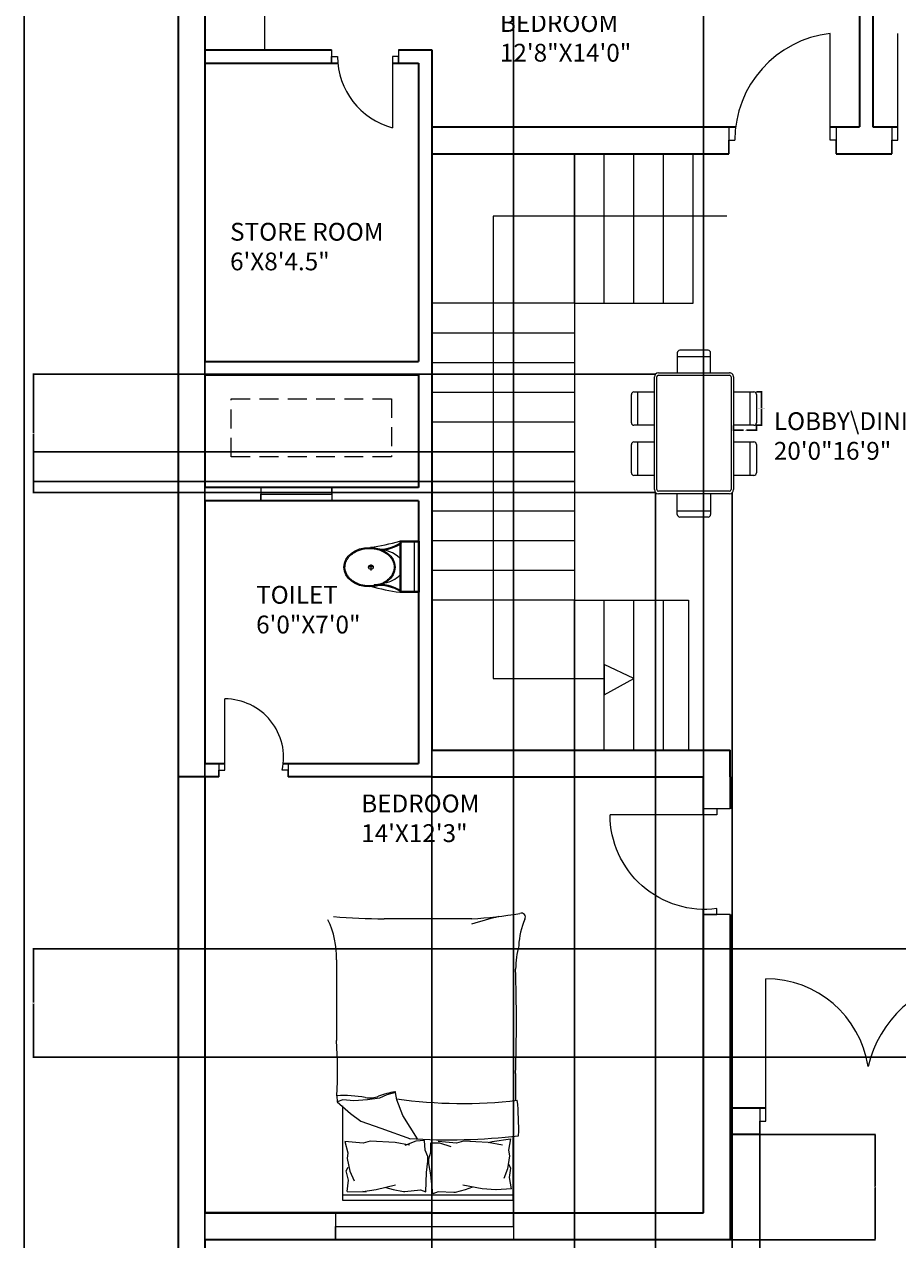
# Model space of a CAD drawing. Units: inches. Extents: x 2460 to 3031, y 933 to 2010.
# Tile 5 of 7: x 2460 to 2754, y 1339 to 1749. Entities that reach past the tile are written whole.
import ezdxf

# ---------------------------------------------------------------- set-up
doc = ezdxf.new("R2010")
doc.units = ezdxf.units.IN
doc.linetypes.add('DASHED2', pattern=[9.525, 6.35, -3.175])
for name, color, linetype, lineweight in [('A-ANNO-DIMS', 2, 'Continuous', 18), ('A-ANNO-SYMB', 7, 'Continuous', 13), ('A-ANNO-TTLB', 7, 'Continuous', 25), ('A-AREA-IDEN', 7, 'Continuous', 18), ('A-DOOR', 4, 'Continuous', 18), ('A-FLOR-CASE', 9, 'Continuous', 18), ('A-FLOR-FIXT', 8, 'Continuous', 18), ('A-FLOR-OVHD', 254, 'DASHED2', 13), ('A-FLOR-STRS', 7, 'Continuous', 18), ('A-FURN', 8, 'Continuous', 18), ('A-GLAZ', 4, 'Continuous', 18), ('A-WALL', 7, 'Continuous', 35), ('C-PROP', 7, 'Continuous', 35)]:
    doc.layers.add(name, color=color, linetype=linetype, lineweight=lineweight)
doc.styles.get("Standard").update_dxf_attribs({"font": 'arial.ttf'})
doc.dimstyles.get("Standard").update_dxf_attribs({"dimtxt": 0.18, "dimasz": 0.18, "dimexe": 0.18, "dimexo": 0.0625, "dimgap": 0.09, "dimtad": 0, "dimtih": 1, "dimtoh": 1, "dimdec": 4, "dimzin": 0, "dimdsep": 46, "dimtxsty": 'Standard', "dimcen": 0.09, "dimadec": 0, "dimazin": 0, "dimtfac": 1, "dimtdec": 4, "dimtofl": 0, "dimtmove": 0, "dimatfit": 3, "dimfxl": 1, "dimtolj": 1, "dimtzin": 0, "dimarcsym": 0})

# ---------------------------------------------------------------- blocks, each defined once
blk = doc.blocks.new('A$C31115884')
for p, q in [((283, 498), (223, 498)), ((258, 466), (258, 523)), ((0, 200), (0, 0)), ((520, 200), (0, 200)), ((10, 190), (10, 10)), ((510, 190), (10, 190)), ((510, 10), (510, 190)), ((520, 0), (520, 200)), ((510, 54), (0, 54)), ((10, 10), (510, 10)), ((0, 0), (520, 0))]:
    blk.add_line(p, q)
blk.add_circle((256, 496), 23.6)
for centre, radius, start, end in [((2778, -205), 2807, 165.4549, 171.7133), ((3237, 905), 2807, 188.2867, 194.5451), ((-295, 403), 365, 324.2091, 9.3499), ((-295, 403), 375, 324.2091, 9.3499), ((139, 406), 293, 315.8436, 2.6563), ((806, 403), 375, 179.2036, 215.7909), ((806, 403), 365, 170.6501, 215.7909), ((384, 406), 293, 190.2774, 224.1564)]:
    blk.add_arc(centre, radius, start, end)
blk.add_ellipse((256, 510), major_axis=(0, -261), ratio=0.772727)
blk.add_open_spline([(256, 259), (263, 259), (270, 260), (288, 262), (299, 265), (320, 273), (330, 278), (350, 291), (360, 299), (378, 316), (386, 326), (402, 347), (409, 358), (421, 383), (427, 395), (436, 422), (440, 436), (445, 465), (447, 480), (448, 509), (448, 524), (445, 553), (443, 568), (436, 596), (432, 610), (422, 636), (416, 649), (402, 672), (395, 683), (379, 703), (370, 712), (351, 728), (341, 735), (321, 746), (310, 751), (289, 757), (278, 759), (256, 761), (245, 761), (223, 757), (212, 754), (191, 746), (181, 741), (161, 728), (151, 720), (133, 703), (125, 693), (110, 672), (103, 660), (90, 636), (85, 623), (76, 596), (72, 582), (67, 553), (66, 538), (64, 509), (65, 494), (68, 465), (70, 450), (77, 422), (81, 408), (91, 382), (97, 370), (111, 346), (118, 335), (135, 316), (144, 307), (162, 291), (172, 284), (193, 273), (203, 269), (225, 262), (236, 260), (250, 259), (253, 259), (256, 259)], degree=3, knots=[0, 0, 0, 0, 0.110105, 0.110105, 0.285049, 0.285049, 0.459994, 0.459994, 0.634938, 0.634938, 0.809882, 0.809882, 0.984827, 0.984827, 1.159771, 1.159771, 1.334715, 1.334715, 1.50966, 1.50966, 1.684604, 1.684604, 1.859549, 1.859549, 2.034493, 2.034493, 2.209437, 2.209437, 2.384382, 2.384382, 2.559326, 2.559326, 2.73427, 2.73427, 2.909215, 2.909215, 3.084159, 3.084159, 3.259103, 3.259103, 3.434048, 3.434048, 3.608992, 3.608992, 3.783936, 3.783936, 3.958881, 3.958881, 4.133825, 4.133825, 4.30877, 4.30877, 4.483714, 4.483714, 4.658658, 4.658658, 4.833603, 4.833603, 5.008547, 5.008547, 5.183491, 5.183491, 5.358436, 5.358436, 5.53338, 5.53338, 5.708324, 5.708324, 5.883269, 5.883269, 6.058213, 6.058213, 6.233158, 6.233158, 6.283185, 6.283185, 6.283185, 6.283185])
blk = doc.blocks.new('BED-DOUBLE')
for p, q in [((75.16, 62.38), (96.87, 62.38)), ((76.95, 55.42), (76.08, 61.53)), ((76.08, 61.53), (79.9, 60.84)), ((85.96, 61.71), (84.75, 61.01)), ((89.08, 61.19), (85.96, 61.71)), ((92.9, 61.88), (89.08, 61.19)), ((92.87, 61.87), (93.27, 56.74)), ((95.03, 62.38), (95.03, 5.09)), ((96.87, 62.38), (96.87, 5.09)), ((78.14, 58.9), (77.34, 54.06)), ((79.9, 60.84), (81.8, 61.19)), ((81.8, 61.19), (86.14, 60.49)), ((86.14, 60.49), (89.43, 59.28)), ((77.34, 54.06), (76.82, 45.66)), ((77.34, 54.06), (76.95, 55.42)), ((93.24, 56.62), (92.9, 52.03)), ((93.27, 56.74), (93.24, 56.62)), ((92.9, 52.03), (91.68, 45.45)), ((1.87, 48.49), (1.87, 18.98)), ((76.82, 45.66), (77.49, 43.31)), ((92.38, 48.74), (93.24, 46.31)), ((93.24, 46.31), (94.11, 42.85)), ((77.49, 43.31), (77, 37.16)), ((77.37, 37.65), (78.68, 41.42)), ((94.11, 42.46), (93.94, 37.13)), ((94.11, 42.85), (94.11, 42.46)), ((77.37, 34.71), (77.37, 37.65)), ((93.94, 37.13), (94.63, 35.4)), ((79.83, 32.82), (76.62, 32.62)), ((80.59, 34.71), (77.37, 34.71)), ((82.03, 33.66), (79.83, 32.82)), ((82.84, 34.01), (80.59, 34.71)), ((83.59, 33.75), (82.03, 33.66)), ((84.4, 34.01), (82.84, 34.01)), ((87.44, 33.3), (83.59, 33.75)), ((88.22, 34.71), (84.4, 34.01)), ((93.88, 33.01), (87.44, 33.3)), ((94.63, 35.4), (88.22, 34.71)), ((93.3, 31.24), (93.88, 33.01)), ((76.03, 30.27), (68.25, 25.25)), ((76.62, 32.62), (76.8, 29.68)), ((76.8, 29.68), (78.34, 26)), ((93.81, 25.93), (93.3, 31.24)), ((68.25, 25.25), (62.87, 23.21)), ((72.52, 17.82), (76.03, 27.82)), ((78.14, 27.51), (77.34, 22.68)), ((93.18, 22.03), (93.83, 25.54)), ((93.83, 25.54), (93.81, 25.93)), ((62.87, 23.21), (60.45, 22.84)), ((60.45, 22.84), (61.2, 19.86)), ((77.34, 22.68), (76.82, 14.27)), ((93.19, 16.3), (91.57, 22.8)), ((92.47, 19.55), (93.18, 22.03)), ((61.2, 19.86), (62.31, 17.45)), ((62.31, 17.45), (62.87, 13.37)), ((70.1, 11.14), (72.52, 17.82)), ((62.87, 13.37), (63.24, 8.72)), ((76.82, 14.27), (77.49, 11.92)), ((93.82, 11.75), (93.19, 16.3)), ((93.81, 6.47), (93.92, 12.95)), ((93.92, 12.95), (93.82, 11.75)), ((63.24, 8.72), (62.87, 5.01)), ((67.51, 7.61), (70.1, 11.14)), ((77.49, 11.92), (77, 5.77)), ((86.97, 7.43), (90.18, 8.85)), ((62.87, 5.01), (63.61, 3.17)), ((63.61, 3.17), (67.51, 7.61)), ((96.87, 5.09), (64.97, 5.09)), ((77, 5.77), (80.77, 6.7)), ((80.77, 6.7), (82.69, 6.47)), ((82.69, 6.47), (86.97, 7.43)), ((86.88, 6.21), (85.62, 6.83)), ((89.96, 6.93), (86.88, 6.21)), ((93.81, 6.47), (89.96, 6.93)), ((61.52, 3.07), (63.61, 3.17, 4.64))]:
    blk.add_line(p, q)
for centre, radius, start, end in [((1.3, 65.24), 1.31, 56.1736, 203.4781), ((12.62, 92.52), 28.25, 247.9751, 266.652), ((-143.9, 40.86), 145.97, 2.9958, 9.4091), ((19.53, 98.8), 35.53, 256.0648, 268.9113), ((36.19, -514.68), 578.22, 88.22771, 91.71854), ((59.5, 267.13), 203.94, 268.4762, 271.0082), ((-90.53, 45.26), 154.68, 351.7845, 6.9006), ((72.78, -35.55), 99.87, 88.7218, 95.604), ((-121.38, 40.94), 197.77, 356.0865, 6.7821), ((125.3, 87.2), 127.63, 193.3832, 197.7053), ((60.38, 22.63), 0.221, 70.2464, 181.1377), ((95.1, 29.2), 35.55, 190.6617, 199.8806), ((-157.62, 17.21), 159.5, 354.4998, 0.6351), ((54.83, 14.11), 7.46, 348.6608, 23.7384), ((104.85, 5.01), 43.38, 169.8763, 182.5657), ((14.55, -24.75), 27.65, 87.4714, 116.4681), ((15.56, 5471.89), 5469.02, 270.00217, 270.28689), ((53.34, -151.96), 155.25, 86.9791, 93.8365)]:
    blk.add_arc(centre, radius, start, end)
blk = doc.blocks.new('CHAIR-DINING-SIDE')
for p, q in [((0, 11.24), (6.88, 11.24)), ((5.62, 0), (5.62, 11.24)), ((7.73, 10.4), (7.73, 0.84)), ((6.88, 0), (0, 0))]:
    blk.add_line(p, q)
for centre, start, end in [((6.88, 10.4), 0, 90), ((6.88, 0.84), 270, 0)]:
    blk.add_arc(centre, 0.843, start, end)
blk = doc.blocks.new('DOOR-SWING-36')
for p, q in [((0, 35.65), (9, 35.65)), ((4.5, 35.65), (4.5, 33.65)), ((4.5, 33.65), (40.5, 33.65)), ((4.5, 0), (4.5, 2)), ((0, 0), (9, 0)), ((9, 0), (4.5, 0))]:
    blk.add_line(p, q)
blk.add_arc((8.58, 33.65), 31.92, 262.6481, 0)
blk = doc.blocks.new('WIN-24-PARTITION')
for p, q in [((2.25, 24), (0, 24)), ((0, 24), (4.5, 24)), ((2.25, 0), (2.25, 24)), ((0, 0), (4.5, 0)), ((4.5, 0), (2.25, 0))]:
    blk.add_line(p, q)
blk = doc.blocks.new('WIN-60')
for p, q in [((0, 9), (0, 0)), ((60, 4.5), (60, 9)), ((60, 9), (60, 0)), ((0, 0), (0, 4.5)), ((0, 4.5), (60, 4.5))]:
    blk.add_line(p, q)
blk = doc.blocks.new('*D16')
at = {"layer": 'A-ANNO-DIMS', "color": 0, "lineweight": -2, "transparency": 16777216}
for p, q in [((2706.57, 1625.17), (2708.38, 1625.17)), ((2708.2, 1624.99), (2708.2, 1619.74)), ((2708.2, 1614.12), (2708.2, 1619.37)), ((2706.57, 1613.94), (2708.38, 1613.94))]:
    blk.add_line(p, q, dxfattribs=at)
at = {"layer": 'A-ANNO-DIMS', "color": 0, "transparency": 16777216}
for points in [[(2708.17, 1624.99), (2708.23, 1624.99), (2708.2, 1625.17)], [(2708.17, 1614.12), (2708.23, 1614.12), (2708.2, 1613.94)]]:
    blk.add_solid(points, dxfattribs=at)
at = {"layer": 'Defpoints', "color": 0, "transparency": 16777216}
for p in [(2706.51, 1625.17), (2708.2, 1625.17), (2706.51, 1613.94)]:
    blk.add_point(p, dxfattribs=at)
at = {"layer": 'A-ANNO-DIMS', "color": 0, "transparency": 16777216, "insert": (2708.2, 1619.55), "char_height": 0.18, "attachment_point": 5}
blk.add_mtext('\\A1;SIDE CHAIR 11 TYP.', dxfattribs=at)
blk = doc.blocks.new('*D17')
at = {"layer": 'A-ANNO-DIMS', "color": 0, "lineweight": -2, "transparency": 16777216}
for p, q in [((2698.78, 1613.87), (2698.78, 1612.07)), ((2706.51, 1613.87), (2706.51, 1612.07)), ((2698.96, 1612.25), (2702.19, 1612.25)), ((2706.33, 1612.25), (2703.11, 1612.25))]:
    blk.add_line(p, q, dxfattribs=at)
at = {"layer": 'A-ANNO-DIMS', "color": 0, "transparency": 16777216}
for points in [[(2698.96, 1612.28), (2698.96, 1612.22), (2698.78, 1612.25)], [(2706.33, 1612.28), (2706.33, 1612.22), (2706.51, 1612.25)]]:
    blk.add_solid(points, dxfattribs=at)
at = {"layer": 'Defpoints', "color": 0, "transparency": 16777216}
for p in [(2698.78, 1613.94), (2706.51, 1613.94), (2706.51, 1612.25)]:
    blk.add_point(p, dxfattribs=at)
at = {"layer": 'A-ANNO-DIMS', "color": 0, "transparency": 16777216, "insert": (2702.65, 1612.25), "char_height": 0.18, "attachment_point": 5}
blk.add_mtext('\\A1;8 TYP.', dxfattribs=at)
blk = doc.blocks.new('*D37')
at = {"layer": 'A-ANNO-DIMS', "color": 0, "lineweight": -2, "transparency": 16777216}
for p, q in [((2597.17, 1554.98), (2597.17, 933.16)), ((2645.17, 1554.98), (2645.17, 933.16)), ((2597.35, 933.34), (2620.95, 933.34)), ((2644.99, 933.34), (2621.39, 933.34))]:
    blk.add_line(p, q, dxfattribs=at)
at = {"layer": 'A-ANNO-DIMS', "color": 0, "transparency": 16777216}
for points in [[(2597.35, 933.37), (2597.35, 933.31), (2597.17, 933.34)], [(2644.99, 933.37), (2644.99, 933.31), (2645.17, 933.34)]]:
    blk.add_solid(points, dxfattribs=at)
at = {"layer": 'Defpoints', "color": 0, "transparency": 16777216}
for p in [(2597.17, 1555.05), (2645.17, 1555.05), (2645.17, 933.34)]:
    blk.add_point(p, dxfattribs=at)
at = {"layer": 'A-ANNO-DIMS', "color": 0, "transparency": 16777216, "insert": (2621.17, 933.34), "char_height": 0.18, "attachment_point": 5}
blk.add_mtext('\\A1;48', dxfattribs=at)
blk = doc.blocks.new('*D38')
at = {"layer": 'A-ANNO-DIMS', "color": 0, "lineweight": -2, "transparency": 16777216}
for p, q in [((2672.51, 1591.25), (2672.51, 933.16)), ((2698.37, 1591.25), (2698.37, 933.16)), ((2672.69, 933.34), (2685.04, 933.34)), ((2698.19, 933.34), (2685.83, 933.34))]:
    blk.add_line(p, q, dxfattribs=at)
at = {"layer": 'A-ANNO-DIMS', "color": 0, "transparency": 16777216}
for points in [[(2672.69, 933.37), (2672.69, 933.31), (2672.51, 933.34)], [(2698.19, 933.37), (2698.19, 933.31), (2698.37, 933.34)]]:
    blk.add_solid(points, dxfattribs=at)
at = {"layer": 'Defpoints', "color": 0, "transparency": 16777216}
for p in [(2672.51, 1591.31), (2698.37, 1591.31), (2698.37, 933.34)]:
    blk.add_point(p, dxfattribs=at)
at = {"layer": 'A-ANNO-DIMS', "color": 0, "transparency": 16777216, "insert": (2685.44, 933.34), "char_height": 0.18, "attachment_point": 5}
blk.add_mtext('\\A1;25.87', dxfattribs=at)
blk = doc.blocks.new('*D39')
at = {"layer": 'A-ANNO-DIMS', "color": 0, "lineweight": -2, "transparency": 16777216}
for p, q in [((2672.44, 1631.22), (2462.69, 1631.22)), ((2462.87, 1631.04), (2462.87, 1611.45)), ((2462.87, 1591.49), (2462.87, 1611.08)), ((2672.44, 1591.31), (2462.69, 1591.31))]:
    blk.add_line(p, q, dxfattribs=at)
at = {"layer": 'A-ANNO-DIMS', "color": 0, "transparency": 16777216}
for points in [[(2462.84, 1631.04), (2462.9, 1631.04), (2462.87, 1631.22)], [(2462.84, 1591.49), (2462.9, 1591.49), (2462.87, 1591.31)]]:
    blk.add_solid(points, dxfattribs=at)
at = {"layer": 'Defpoints', "color": 0, "transparency": 16777216}
for p in [(2462.87, 1631.22), (2672.51, 1631.22), (2672.51, 1591.31)]:
    blk.add_point(p, dxfattribs=at)
at = {"layer": 'A-ANNO-DIMS', "color": 0, "transparency": 16777216, "insert": (2462.87, 1611.27), "char_height": 0.18, "attachment_point": 5}
blk.add_mtext('\\A1;39.92', dxfattribs=at)
blk = doc.blocks.new('*D40')
at = {"layer": 'A-ANNO-DIMS', "color": 0, "lineweight": -2, "transparency": 16777216}
for p, q in [((2511.67, 1056.05), (2511.67, 2006.96)), ((2511.85, 2006.78), (2516.02, 2006.78)), ((2520.49, 2006.78), (2516.32, 2006.78)), ((2520.67, 1056.05), (2520.67, 2006.96))]:
    blk.add_line(p, q, dxfattribs=at)
at = {"layer": 'A-ANNO-DIMS', "color": 0, "transparency": 16777216}
for points in [[(2511.85, 2006.81), (2511.85, 2006.75), (2511.67, 2006.78)], [(2520.49, 2006.81), (2520.49, 2006.75), (2520.67, 2006.78)]]:
    blk.add_solid(points, dxfattribs=at)
at = {"layer": 'Defpoints', "color": 0, "transparency": 16777216}
for p in [(2520.67, 2006.78), (2511.67, 1055.98), (2520.67, 1055.98)]:
    blk.add_point(p, dxfattribs=at)
at = {"layer": 'A-ANNO-DIMS', "color": 0, "transparency": 16777216, "insert": (2516.17, 2006.78), "char_height": 0.18, "attachment_point": 5}
blk.add_mtext('\\A1;9', dxfattribs=at)
blk = doc.blocks.new('*D42')
at = {"layer": 'A-ANNO-DIMS', "color": 0, "lineweight": -2, "transparency": 16777216}
for p, q in [((2645.11, 1605.05), (2462.69, 1605.05)), ((2462.87, 1604.87), (2462.87, 1600.23)), ((2462.87, 1595.23), (2462.87, 1599.86)), ((2645.11, 1595.05), (2462.69, 1595.05))]:
    blk.add_line(p, q, dxfattribs=at)
at = {"layer": 'A-ANNO-DIMS', "color": 0, "transparency": 16777216}
for points in [[(2462.84, 1604.87), (2462.9, 1604.87), (2462.87, 1605.05)], [(2462.84, 1595.23), (2462.9, 1595.23), (2462.87, 1595.05)]]:
    blk.add_solid(points, dxfattribs=at)
at = {"layer": 'Defpoints', "color": 0, "transparency": 16777216}
for p in [(2462.87, 1605.05), (2645.17, 1605.05), (2645.17, 1595.05)]:
    blk.add_point(p, dxfattribs=at)
at = {"layer": 'A-ANNO-DIMS', "color": 0, "transparency": 16777216, "insert": (2462.87, 1600.05), "char_height": 0.18, "attachment_point": 5}
blk.add_mtext('\\A1;10', dxfattribs=at)
blk = doc.blocks.new('*D43')
at = {"layer": 'A-ANNO-DIMS', "color": 0, "lineweight": -2, "transparency": 16777216}
for p, q in [((2707.62, 1374.89), (2707.62, 933.16)), ((2778.55, 1374.89), (2778.55, 933.16)), ((2707.8, 933.34), (2742.69, 933.34)), ((2778.37, 933.34), (2743.48, 933.34))]:
    blk.add_line(p, q, dxfattribs=at)
at = {"layer": 'A-ANNO-DIMS', "color": 0, "transparency": 16777216}
for points in [[(2707.8, 933.37), (2707.8, 933.31), (2707.62, 933.34)], [(2778.37, 933.37), (2778.37, 933.31), (2778.55, 933.34)]]:
    blk.add_solid(points, dxfattribs=at)
at = {"layer": 'Defpoints', "color": 0, "transparency": 16777216}
for p in [(2707.62, 1374.95), (2778.55, 1374.95), (2778.55, 933.34)]:
    blk.add_point(p, dxfattribs=at)
at = {"layer": 'A-ANNO-DIMS', "color": 0, "transparency": 16777216, "insert": (2743.09, 933.34), "char_height": 0.18, "attachment_point": 5}
blk.add_mtext('\\A1;70.93', dxfattribs=at)
blk = doc.blocks.new('*D44')
at = {"layer": 'A-ANNO-DIMS', "color": 0, "lineweight": -2, "transparency": 16777216}
for p, q in [((2624.64, 1348.55), (2624.64, 2006.96)), ((2624.82, 2006.78), (2656.26, 2006.78)), ((2688.49, 2006.78), (2657.05, 2006.78)), ((2688.67, 1348.55), (2688.67, 2006.96))]:
    blk.add_line(p, q, dxfattribs=at)
at = {"layer": 'A-ANNO-DIMS', "color": 0, "transparency": 16777216}
for points in [[(2624.82, 2006.81), (2624.82, 2006.75), (2624.64, 2006.78)], [(2688.49, 2006.81), (2688.49, 2006.75), (2688.67, 2006.78)]]:
    blk.add_solid(points, dxfattribs=at)
at = {"layer": 'Defpoints', "color": 0, "transparency": 16777216}
for p in [(2688.67, 2006.78), (2624.64, 1348.48), (2688.67, 1348.48)]:
    blk.add_point(p, dxfattribs=at)
at = {"layer": 'A-ANNO-DIMS', "color": 0, "transparency": 16777216, "insert": (2656.65, 2006.78), "char_height": 0.18, "attachment_point": 5}
blk.add_mtext('\\A1;64.03', dxfattribs=at)
blk = doc.blocks.new('*D50')
at = {"layer": 'A-ANNO-DIMS', "color": 0, "lineweight": -2, "transparency": 16777216}
for p, q in [((2901.55, 1437.46), (2462.69, 1437.46)), ((2462.87, 1437.28), (2462.87, 1419.38)), ((2462.87, 1401.12), (2462.87, 1419.02)), ((2901.55, 1400.94), (2462.69, 1400.94))]:
    blk.add_line(p, q, dxfattribs=at)
at = {"layer": 'A-ANNO-DIMS', "color": 0, "transparency": 16777216}
for points in [[(2462.84, 1437.28), (2462.9, 1437.28), (2462.87, 1437.46)], [(2462.84, 1401.12), (2462.9, 1401.12), (2462.87, 1400.94)]]:
    blk.add_solid(points, dxfattribs=at)
at = {"layer": 'Defpoints', "color": 0, "transparency": 16777216}
for p in [(2462.87, 1437.46), (2901.62, 1437.46), (2901.62, 1400.94)]:
    blk.add_point(p, dxfattribs=at)
at = {"layer": 'A-ANNO-DIMS', "color": 0, "transparency": 16777216, "insert": (2462.87, 1419.2), "char_height": 0.18, "attachment_point": 5}
blk.add_mtext('\\A1;36.524', dxfattribs=at)
blk = doc.blocks.new('*D51')
at = {"layer": 'A-ANNO-DIMS', "color": 0, "lineweight": -2, "transparency": 16777216}
for p, q in [((2697.73, 1374.95), (2746.65, 1374.95)), ((2746.47, 1374.77), (2746.47, 1357.4)), ((2746.47, 1339.66), (2746.47, 1357.03)), ((2697.73, 1339.48), (2746.65, 1339.48))]:
    blk.add_line(p, q, dxfattribs=at)
at = {"layer": 'A-ANNO-DIMS', "color": 0, "transparency": 16777216}
for points in [[(2746.44, 1374.77), (2746.5, 1374.77), (2746.47, 1374.95)], [(2746.44, 1339.66), (2746.5, 1339.66), (2746.47, 1339.48)]]:
    blk.add_solid(points, dxfattribs=at)
at = {"layer": 'Defpoints', "color": 0, "transparency": 16777216}
for p in [(2697.67, 1374.95), (2697.67, 1339.48), (2746.47, 1339.48)]:
    blk.add_point(p, dxfattribs=at)
at = {"layer": 'A-ANNO-DIMS', "color": 0, "transparency": 16777216, "insert": (2746.47, 1357.22), "char_height": 0.18, "attachment_point": 5}
blk.add_mtext('\\A1;35.466', dxfattribs=at)

msp = doc.modelspace()

# ---------------------------------------------------------------- linework, layer by layer
at = {"layer": 'A-ANNO-SYMB'}
for p, q in [((2696.5623, 1684.4614), (2617.8347, 1684.4614)), ((2617.8347, 1684.4614), (2617.8347, 1528.6315)), ((2665.1684, 1528.6315), (2655.1684, 1533.301)), ((2655.1684, 1533.301), (2655.1684, 1523.12)), ((2617.8347, 1528.6315), (2655.1684, 1528.6315)), ((2655.1684, 1523.12), (2665.1684, 1528.6315))]:
    msp.add_line(p, q, dxfattribs=at)
at = {"layer": 'A-ANNO-TTLB'}
msp.add_lwpolyline([(2459.8083, 2009.7942), (3030.6598, 2009.7942), (3030.6598, 936.3732), (2459.8083, 936.3732)], close=True, dxfattribs=at)
at = {"layer": 'A-DOOR'}
for p, q in [((2731.3312, 1709.9828), (2731.3312, 1745.9828)), ((2754.0876, 1709.9828), (2754.0876, 1745.9828)), ((2563.3673, 1740.4828), (2563.3673, 1735.9828)), ((2563.3673, 1735.9828), (2563.3673, 1738.2328)), ((2563.3673, 1738.2328), (2565.3673, 1738.2328)), ((2585.907, 1738.2328), (2583.907, 1738.2328)), ((2583.907, 1738.2328), (2583.907, 1714.2328)), ((2585.907, 1740.4828), (2585.907, 1735.9828)), ((2585.907, 1735.9828), (2585.907, 1738.2328)), ((2697.2049, 1714.4828), (2697.2049, 1705.4828)), ((2733.3312, 1714.4828), (2733.3312, 1705.4828)), ((2752.0876, 1714.4828), (2752.0876, 1705.4828)), ((2697.2049, 1705.4828), (2697.2049, 1709.9828)), ((2697.2049, 1709.9828), (2699.2049, 1709.9828)), ((2733.3312, 1709.9828), (2731.3312, 1709.9828)), ((2733.3312, 1705.4828), (2733.3312, 1709.9828)), ((2752.0876, 1705.4828), (2752.0876, 1709.9828)), ((2752.0876, 1709.9828), (2754.0876, 1709.9828)), ((2527.3672, 1497.7328), (2527.3672, 1521.7328)), ((2525.3672, 1499.9828), (2525.3672, 1495.4828)), ((2548.7319, 1499.9828), (2548.7319, 1495.4828)), ((2525.3672, 1495.4828), (2525.3672, 1497.7328)), ((2525.3672, 1497.7328), (2527.3672, 1497.7328)), ((2548.7319, 1497.7328), (2546.7319, 1497.7328)), ((2548.7319, 1495.4828), (2548.7319, 1497.7328)), ((2709.6216, 1415.4491), (2709.6216, 1427.4491)), ((2709.6216, 1379.4491), (2709.6216, 1415.4491)), ((2707.6216, 1383.9491), (2707.6216, 1374.9491)), ((2707.6216, 1374.9491), (2707.6216, 1379.4491)), ((2707.6216, 1379.4491), (2709.6216, 1379.4491))]:
    msp.add_line(p, q, dxfattribs=at)
for centre, radius, start, end in [((2735.4384, 1709.9828), 36.2335, 96.508647, 180), ((2590.1713, 1738.2328), 24.8041, 180, 255.371471), ((2527.3672, 1501.9205), 19.8123, 347.797364, 90), ((2709.6216, 1392.5701), 34.879, 8.735664, 90), ((2781.8372, 1389.0544), 38.7565, 97.834609, 166.856265)]:
    msp.add_arc(centre, radius, start, end, dxfattribs=at)
at = {"layer": 'A-FLOR-CASE'}
msp.add_line((2540.7485, 1842.4828), (2540.7485, 1740.4828), dxfattribs=at)
at = {"layer": 'A-FLOR-OVHD'}
msp.add_lwpolyline([(2529.5594, 1622.8177), (2583.5305, 1622.8177), (2583.5305, 1603.3491), (2529.5594, 1603.3491)], close=True, dxfattribs=at)
at = {"layer": 'A-FLOR-STRS'}
for p, q in [((2645.1684, 1705.4828), (2645.1684, 1655.0454)), ((2645.1684, 1655.0454), (2645.1684, 1705.4828)), ((2655.1684, 1655.0454), (2655.1684, 1705.4828)), ((2665.1684, 1655.0454), (2665.1684, 1705.4828)), ((2675.1684, 1655.0454), (2675.1684, 1705.4828)), ((2685.1684, 1655.0454), (2685.1684, 1705.4828)), ((2645.1684, 1655.0454), (2597.1684, 1655.0454)), ((2645.1684, 1657.4828), (2645.1684, 1552.4828)), ((2645.1684, 1655.0454), (2685.1684, 1655.0454)), ((2645.1684, 1645.0454), (2597.1684, 1645.0454)), ((2645.1684, 1635.0454), (2597.1684, 1635.0454)), ((2645.1684, 1625.0454), (2597.1684, 1625.0454)), ((2645.1684, 1615.0454), (2597.1684, 1615.0454)), ((2645.1684, 1605.0454), (2597.1684, 1605.0454)), ((2645.1684, 1595.0454), (2597.1684, 1595.0454)), ((2645.1684, 1585.0454), (2597.1684, 1585.0454)), ((2645.1684, 1575.0454), (2597.1684, 1575.0454)), ((2645.1684, 1565.0454), (2597.1684, 1565.0454)), ((2645.1684, 1555.0454), (2597.1684, 1555.0454)), ((2597.1684, 1504.4828), (2597.1684, 1552.4828)), ((2645.1684, 1555.0454), (2645.1684, 1504.4828)), ((2645.1684, 1504.4828), (2645.1684, 1555.0454)), ((2645.1684, 1555.0454), (2683.6492, 1555.0454)), ((2655.1684, 1504.4828), (2655.1684, 1555.0454)), ((2665.1684, 1504.4828), (2665.1684, 1555.0454)), ((2675.1684, 1504.4828), (2675.1684, 1555.0454)), ((2683.6492, 1555.0454), (2683.6492, 1504.4828))]:
    msp.add_line(p, q, dxfattribs=at)
at = {"layer": 'A-FURN'}
for p, q in [((2690.2157, 1639.2221), (2680.663, 1639.2221)), ((2679.8201, 1638.3792), (2679.8201, 1631.6361)), ((2679.8201, 1637.1148), (2691.0585, 1637.1148)), ((2691.0585, 1631.6361), (2691.0585, 1638.3792)), ((2672.0936, 1592.3014), (2672.0936, 1630.2313)), ((2672.9365, 1592.3014), (2672.9365, 1630.2313)), ((2673.4985, 1631.6361), (2697.3802, 1631.6361)), ((2673.4985, 1630.7932), (2697.3802, 1630.7932)), ((2697.9421, 1630.2313), (2697.9421, 1592.3015)), ((2698.785, 1630.2313), (2698.785, 1592.3015)), ((2697.3802, 1591.7396), (2673.4985, 1591.7396)), ((2697.3802, 1590.8967), (2673.4985, 1590.8967)), ((2679.8201, 1583.8726), (2679.8201, 1590.8967)), ((2691.0585, 1590.8967), (2691.0585, 1583.8726)), ((2679.8201, 1585.137), (2691.0585, 1585.137)), ((2690.2157, 1583.0297), (2680.663, 1583.0297))]:
    msp.add_line(p, q, dxfattribs=at)
for centre, radius, start, end in [((2680.663, 1638.3792), 0.8429, 90, 180), ((2690.2157, 1638.3792), 0.8429, 0, 90), ((2673.4985, 1630.2313), 1.4048, 90.000003, 180), ((2673.4985, 1630.2313), 0.5619, 90.000003, 180), ((2697.3802, 1630.2313), 1.4048, 0, 90.00001), ((2697.3802, 1630.2313), 0.5619, 0, 90.00001), ((2673.4985, 1592.3014), 1.4048, 180, 270), ((2673.4985, 1592.3014), 0.5619, 180, 270), ((2697.3802, 1592.3015), 1.4048, 270, 0), ((2697.3802, 1592.3015), 0.5619, 270, 0), ((2680.663, 1583.8726), 0.8429, 180, 270), ((2690.2157, 1583.8726), 0.8429, 270, 0)]:
    msp.add_arc(centre, radius, start, end, dxfattribs=at)
at = {"layer": 'A-WALL'}
for p, q in [((2741.1684, 1890.4828), (2741.1684, 1714.4828)), ((2745.6684, 1890.4828), (2745.6684, 1714.4828)), ((2520.6684, 1842.4828), (2520.6684, 1635.4828)), ((2520.6684, 1740.4828), (2563.3673, 1740.4828)), ((2585.907, 1740.4828), (2592.6684, 1740.4828)), ((2592.6684, 1740.4828), (2597.1684, 1740.4828)), ((2597.1684, 1740.4828), (2597.1684, 1504.4828)), ((2520.6684, 1735.9828), (2565.4695, 1735.9828)), ((2583.907, 1735.9828), (2592.6684, 1735.9828)), ((2592.6684, 1735.9828), (2592.6684, 1635.4828)), ((2597.1684, 1714.4828), (2699.4854, 1714.4828)), ((2731.3312, 1714.4828), (2741.1684, 1714.4828)), ((2745.6684, 1714.4828), (2754.0876, 1714.4828)), ((2597.1684, 1705.4828), (2697.2049, 1705.4828)), ((2733.3312, 1705.4828), (2752.0876, 1705.4828)), ((2520.6684, 1635.4828), (2592.6684, 1635.4828)), ((2520.6684, 1630.9828), (2592.6684, 1630.9828)), ((2520.6684, 1630.9828), (2520.6684, 1592.9828)), ((2592.6684, 1630.9828), (2592.6684, 1592.9828)), ((2592.6684, 1592.9828), (2520.6684, 1592.9828)), ((2592.6684, 1588.4828), (2520.6684, 1588.4828)), ((2520.6684, 1588.4828), (2520.6684, 1499.9828)), ((2592.6684, 1588.4828), (2592.6684, 1499.9828)), ((2597.1684, 1504.4828), (2697.6684, 1504.4828)), ((2697.6684, 1495.4828), (2697.6684, 1504.4828)), ((2520.6684, 1499.9828), (2527.3672, 1499.9828)), ((2547.0845, 1499.9828), (2592.6684, 1499.9828)), ((2525.3672, 1495.4828), (2511.6684, 1495.4828)), ((2520.6684, 1495.4828), (2520.6684, 1348.4828)), ((2597.1684, 1495.4828), (2548.7319, 1495.4828)), ((2597.1684, 1495.4828), (2688.6684, 1495.4828)), ((2688.6684, 1482.7065), (2688.6684, 1495.4828)), ((2697.6684, 1495.4828), (2697.6684, 1484.7065)), ((2688.6684, 1348.4828), (2688.6684, 1450.7932)), ((2697.6684, 1449.0529), (2697.6684, 1348.4828)), ((2697.6684, 1383.9491), (2709.6216, 1383.9491)), ((2707.6216, 1374.9491), (2697.6684, 1374.9491)), ((2597.1684, 1348.4828), (2520.6684, 1348.4828)), ((2520.6684, 1348.4828), (2688.6684, 1348.4828)), ((2697.6684, 1348.4828), (2697.6684, 1339.4828)), ((2597.1684, 1339.4828), (2520.6684, 1339.4828)), ((2697.6684, 1339.4828), (2597.1684, 1339.4828))]:
    msp.add_line(p, q, dxfattribs=at)
at = {"layer": 'C-PROP'}
for p, q in [((2511.6684, 1957.9828), (2511.6684, 1055.9828)), ((2511.6684, 1957.9828), (2511.6684, 1055.9828)), ((2520.6684, 1339.4828), (2520.6684, 1055.9828))]:
    msp.add_line(p, q, dxfattribs=at)

# ---------------------------------------------------------------- block references
at = {"layer": 'A-DOOR', "extrusion": (0, 0, -1), "zscale": -1}
msp.add_blockref('DOOR-SWING-36', (-2697.6689, 1449.053), dxfattribs=at)
at = {"layer": 'A-FLOR-FIXT', "xscale": 0.0330640103915726, "yscale": 0.0330640103915726, "zscale": 0.0330640103915726, "rotation": 89.99999999999991}
msp.add_blockref('A$C31115884', (2592.9991, 1557.6589), dxfattribs=at)
at = {"layer": 'A-FURN'}
for name, p, rotation in [('CHAIR-DINING-SIDE', (2672.0936, 1625.1735), 180), ('CHAIR-DINING-SIDE', (2672.0936, 1608.3158), 180), ('BED-DOUBLE', (2562.0769, 1449.532), 269.9999999999999)]:
    msp.add_blockref(name, p, dxfattribs=dict(at, rotation=rotation))
for p in [(2698.785, 1613.936), (2698.785, 1597.0783)]:
    msp.add_blockref('CHAIR-DINING-SIDE', p, dxfattribs=at)
at = {"layer": 'A-GLAZ', "rotation": 269.9999999999994}
msp.add_blockref('WIN-24-PARTITION', (2539.464, 1592.9832), dxfattribs=at)
at = {"layer": 'A-GLAZ'}
msp.add_blockref('WIN-60', (2564.639, 1339.483), dxfattribs=at)

# ---------------------------------------------------------------- texts
at = {"layer": 'A-AREA-IDEN', "char_height": 6, "attachment_point": 1}
for s, width, insert in [('BEDROOM\\P12\'8"X14\'0"', 68.258258, (2620.0635, 1752.504)), ('STORE ROOM \\P6\'X8\'4.5"', 95.089329, (2529.14, 1682.1647)), ('LOBBY\\\\DINING AREA\\P20\'0"16\'9"', 152.675752, (2712.3561, 1618.3354)), ('TOILET \\P6\'0"X7\'0"', 70.247809, (2537.9156, 1559.8037)), ('BEDROOM\\P14\'X12\'3"', 117.6505, (2573.3285, 1489.4952))]:
    msp.add_mtext_dynamic_manual_height_columns(s, width=width, gutter_width=12.5, heights=[0], dxfattribs=dict(at, insert=insert))

# ---------------------------------------------------------------- dimensions: what is measured, and where the dimension line sits
at = {"layer": 'A-ANNO-DIMS'}
for base, p1, p2, override, picture, middle in [((2520.6684, 2006.7823), (2511.6684, 1055.9828), (2520.6684, 1055.9828), {"dimdec": 0, "dimlfac": 1, "dimrnd": 0, "dimzin": 0, "dimdsep": 46, "dimlunit": 2}, '*D40', (2516.1684, 2006.7823)), ((2688.6684, 2006.7823), (2624.6394, 1348.4828), (2688.6684, 1348.4828), {"dimdec": 2, "dimlfac": 1, "dimrnd": 0, "dimzin": 0, "dimdsep": 46, "dimlunit": 2}, '*D44', (2656.6539, 2006.7823)), ((2698.3735, 933.3411), (2672.5051, 1591.3081), (2698.3735, 1591.3082), {"dimdec": 2, "dimlfac": 1, "dimrnd": 0, "dimzin": 0, "dimdsep": 46, "dimlunit": 2}, '*D38', (2685.4393, 933.3411)), ((2645.1684, 933.3411), (2597.1684, 1555.0454), (2645.1684, 1555.0454), {"dimdec": 0, "dimlfac": 1, "dimrnd": 0, "dimzin": 0, "dimdsep": 46, "dimlunit": 2}, '*D37', (2621.1684, 933.3411)), ((2778.5542, 933.3411), (2707.6216, 1374.9491), (2778.5542, 1374.9491), {"dimdec": 2, "dimlfac": 1, "dimrnd": 0, "dimzin": 0, "dimdsep": 46, "dimlunit": 2}, '*D43', (2743.0879, 933.3411))]:
    dim = msp.add_linear_dim(base=base, p1=p1, p2=p2, dimstyle='Standard', override=override, dxfattribs=at)
    dim.commit()
    dim.dimension.update_dxf_attribs({"geometry": picture, "text_midpoint": middle})
for base, p1, p2, angle, override, picture, middle in [((2462.8689, 1631.2247), (2672.5051, 1591.3081), (2672.5051, 1631.2247), 90, {"dimdec": 2, "dimlfac": 1, "dimrnd": 0, "dimzin": 0, "dimdsep": 46, "dimlunit": 2}, '*D39', (2462.8689, 1611.2664)), ((2462.8689, 1605.0454), (2645.1684, 1595.0454), (2645.1684, 1605.0454), 90, {"dimdec": 0, "dimlfac": 1, "dimrnd": 0, "dimzin": 0, "dimdsep": 46, "dimlunit": 2}, '*D42', (2462.8689, 1600.0454)), ((2462.86893, 1437.45968), (2901.61619, 1400.93524), (2901.61619, 1437.45968), 90, {"dimdec": 3, "dimlfac": 1, "dimrnd": 0, "dimzin": 0, "dimdsep": 46, "dimlunit": 2}, '*D50', (2462.86893, 1419.19746)), ((2746.4679, 1339.4828), (2697.6684, 1374.9491), (2697.6684, 1339.4828), 270, {"dimdec": 3, "dimlfac": 1, "dimrnd": 0, "dimzin": 0, "dimdsep": 46, "dimlunit": 2}, '*D51', (2746.4679, 1357.216))]:
    dim = msp.add_linear_dim(base=base, p1=p1, p2=p2, angle=angle, dimstyle='Standard', override=override, dxfattribs=at)
    dim.commit()
    dim.dimension.update_dxf_attribs({"geometry": picture, "text_midpoint": middle})
dim = msp.add_linear_dim(base=(2708.1972, 1625.174), p1=(2706.5115, 1613.9355), p2=(2706.5115, 1625.174), angle=90, text='SIDE CHAIR <> TYP.', dimstyle='Standard', override={"dimdec": 0, "dimlfac": 1, "dimrnd": 0, "dimzin": 0, "dimdsep": 46, "dimlunit": 2}, dxfattribs=at)
dim.commit()
dim.dimension.update_dxf_attribs({"geometry": '*D16', "text_midpoint": (2708.1972, 1619.5548)})
dim = msp.add_linear_dim(base=(2706.5115, 1612.2498), p1=(2698.785, 1613.9355), p2=(2706.5115, 1613.9355), text='<> TYP.', dimstyle='Standard', override={"dimdec": 0, "dimlfac": 1, "dimrnd": 0, "dimzin": 0, "dimdsep": 46, "dimlunit": 2}, dxfattribs=at)
dim.commit()
dim.dimension.update_dxf_attribs({"geometry": '*D17', "text_midpoint": (2702.6482, 1612.2498)})

doc.saveas('drawing.dxf')
